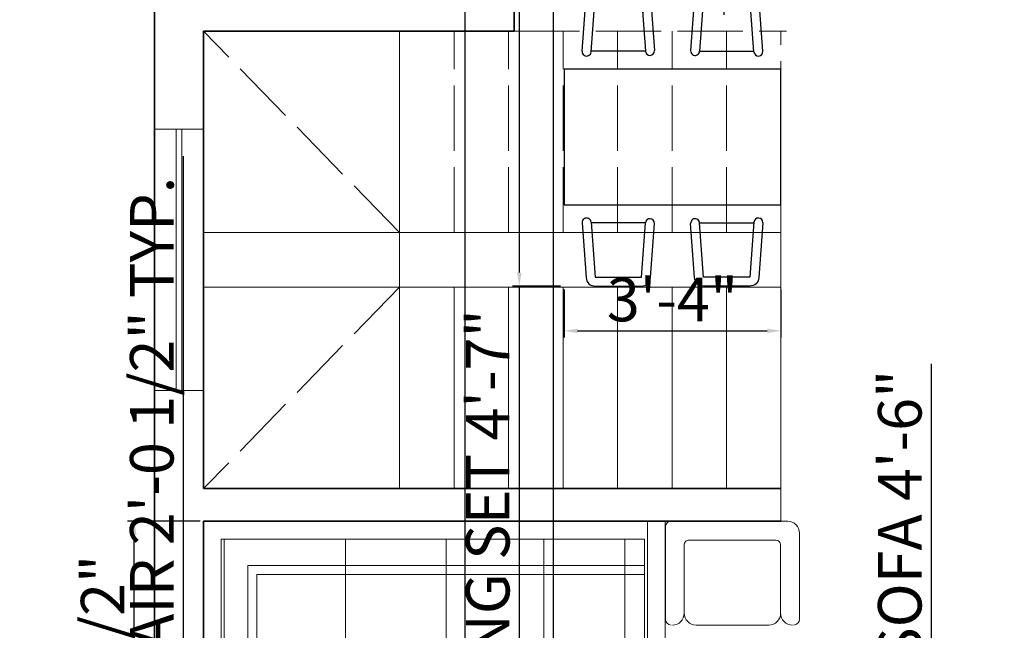
# Model space of a CAD drawing. Units: inches. Extents: x 3394 to 4794, y 965 to 1718.
# Tile 7 of 15: x 3523 to 3704, y 1338 to 1450. Entities that reach past the tile are written whole.
import ezdxf

# ---------------------------------------------------------------- set-up
doc = ezdxf.new("R2010")
doc.units = ezdxf.units.IN
doc.linetypes.add('ACAD_ISO02W100', pattern=[15, 12, -3])
for name, color, linetype, lineweight in [('A-ANNO-DIMS', 2, 'Continuous', 13), ('A-FLOR-STRS', 7, 'Continuous', 18), ('A-FLOR-STRS-OVHD', 7, 'ACAD_ISO02W100', 13), ('A-GLAZ', 4, 'Continuous', 18), ('A-WALL', 7, 'Continuous', 35), ('NOITHAT', 21, 'Continuous', 18)]:
    doc.layers.add(name, color=color, linetype=linetype, lineweight=lineweight)
doc.layers.add('NOI THAT', color=42, linetype='Continuous')
doc.styles.get("Standard").update_dxf_attribs({"font": 'arial.ttf'})
doc.dimstyles.new('ISO-25', dxfattribs={"dimtxt": 8, "dimasz": 2.5, "dimexe": 1.25, "dimexo": 0.625, "dimtad": 1, "dimlunit": 3, "dimtxsty": 'Standard', "dimcen": 2.5, "dimadec": 0, "dimazin": 0, "dimtfac": 1, "dimtmove": 0, "dimatfit": 3, "dimfxl": 1, "dimarcsym": 0})

# ---------------------------------------------------------------- blocks, each defined once
blk = doc.blocks.new('sofa-27')
at = {"color": 0, "linetype": 'ByBlock'}
for p, q in [((0.0945, 0.5198), (0.459, 0.5198)), ((-0.0591, 0.0591), (-0.0591, 0.4902)), ((0.0354, 0.1181), (0.0354, 0.4607)), ((0.518, 0.1181), (0.518, 0.4607)), ((0.6125, 0.0295), (0.6125, 0.4902)), ((0.4944, 0.0945), (0.0591, 0.0945)), ((0.583, 0), (0, 0))]:
    blk.add_line(p, q, dxfattribs=at)
for centre, radius, start, end in [((-0.0295, 0.4902), 0.0295, 90, 180), ((-0.0236, 0.4607), 0.0591, 360, 90), ((0.0945, 0.4607), 0.0591, 90, 180), ((0.459, 0.4607), 0.0591, 0, 90), ((0.5771, 0.4607), 0.0591, 90, 180), ((0.583, 0.4902), 0.0295, 0, 90), ((0.0591, 0.1181), 0.0236, 180, 270), ((0.4944, 0.1181), 0.0236, 270, 0), ((0, 0.0591), 0.0591, 180, 270), ((0.583, 0.0295), 0.0295, 270, 0)]:
    blk.add_arc(centre, radius, start, end, dxfattribs=at)
blk = doc.blocks.new('TABLE-30A')
at = {"color": 0, "linetype": 'ByBlock'}
for p, q in [((0, 0), (0, 0.55)), ((0, 0.55), (1.5, 0.55)), ((1.5, 0.55), (1.5, 0)), ((0.051, 0.508), (0.042, 0.499)), ((0.042, 0.499), (0.042, 0.478)), ((0.042, 0.478), (0.072, 0.478)), ((0.042, 0.478), (0.042, 0.41)), ((0.072, 0.508), (0.051, 0.508)), ((0.051, 0.478), (0.051, 0.41)), ((0.072, 0.478), (0.072, 0.508)), ((0.072, 0.508), (0.14, 0.508)), ((0.072, 0.499), (0.14, 0.499)), ((1.331, 0.508), (0.169, 0.508)), ((1.331, 0.499), (0.169, 0.499)), ((1.428, 0.508), (1.36, 0.508)), ((1.428, 0.499), (1.36, 0.499)), ((1.428, 0.508), (1.428, 0.478)), ((1.449, 0.508), (1.428, 0.508)), ((1.428, 0.478), (1.458, 0.478)), ((1.458, 0.499), (1.449, 0.508)), ((1.449, 0.478), (1.449, 0.41)), ((1.458, 0.478), (1.458, 0.499)), ((1.458, 0.478), (1.458, 0.41)), ((0.042, 0.169), (0.042, 0.381)), ((0.051, 0.169), (0.051, 0.381)), ((1.449, 0.381), (1.449, 0.169)), ((1.458, 0.381), (1.458, 0.169)), ((0.042, 0.072), (0.042, 0.14)), ((0.051, 0.072), (0.051, 0.14)), ((1.449, 0.072), (1.449, 0.14)), ((1.458, 0.072), (1.458, 0.14)), ((1.5, 0), (0, 0)), ((0.042, 0.072), (0.042, 0.051)), ((0.072, 0.072), (0.042, 0.072)), ((0.042, 0.051), (0.051, 0.042)), ((0.051, 0.042), (0.072, 0.042)), ((0.072, 0.042), (0.072, 0.072)), ((0.072, 0.051), (0.14, 0.051)), ((0.072, 0.042), (0.14, 0.042)), ((0.169, 0.051), (1.331, 0.051)), ((0.169, 0.042), (1.331, 0.042)), ((1.428, 0.051), (1.36, 0.051)), ((1.428, 0.042), (1.36, 0.042)), ((1.428, 0.072), (1.428, 0.042)), ((1.458, 0.072), (1.428, 0.072)), ((1.428, 0.042), (1.449, 0.042)), ((1.449, 0.042), (1.458, 0.051)), ((1.458, 0.051), (1.458, 0.072))]:
    blk.add_line(p, q, dxfattribs=at)
blk = doc.blocks.new('12')
at = {"color": 0}
for p, q in [((5656.26, 3021.25), (5553.9, 3021.25)), ((5553.9, 3021.25), (5553.9, 2989.76)), ((5557.83, 3021.25), (5557.83, 2989.76)), ((5656.26, 2989.76), (5656.26, 3021.25)), ((5652.32, 3017.31), (5558.49, 3017.31)), ((5558.49, 3017.31), (5558.49, 2989.76)), ((5562.89, 3017.31), (5562.89, 2989.76)), ((5580.8, 3017.31), (5580.8, 2989.76)), ((5602.45, 3017.31), (5602.45, 2989.76)), ((5624.76, 3017.31), (5624.76, 2954.53)), ((5651.66, 3017.31), (5651.66, 2954.53)), ((5652.32, 2989.76), (5652.32, 3017.31)), ((5646.42, 3011.41), (5558.49, 3011.41)), ((5646.42, 2954.53), (5646.42, 3011.41)), ((5644.45, 3009.44), (5558.49, 3009.44)), ((5644.45, 2954.53), (5644.45, 3009.44)), ((5624.76, 2995), (5624.76, 2954.53)), ((5558.49, 2989.76), (5624.76, 2989.76)), ((5651.66, 2954.53), (5624.76, 2954.53))]:
    blk.add_line(p, q, dxfattribs=at)
for centre in [(5555.86, 2989.76), (5654.29, 2989.76)]:
    blk.add_arc(centre, 1.97, 180, 0, dxfattribs=at)
at = {"xscale": -20.70834898381633, "yscale": 20.70834898381633, "zscale": 20.70834898381633}
blk.add_blockref('TABLE-30A', (5601.8, 2960.82), dxfattribs=at)
blk = doc.blocks.new('A$C02103572')
at = {"layer": 'NOI THAT'}
for p, q in [((450, 1200), (450, 0)), ((1200, 1200), (450, 1200)), ((1200, 0), (1200, 1200)), ((350, 750.1), (350, 1049.9)), ((1300, 750.1), (1300, 1049.9)), ((350, 449.9), (350, 150.1)), ((1300, 449.9), (1300, 150.1)), ((450, 0), (1200, 0))]:
    blk.add_line(p, q, dxfattribs=at)
for points in [[(350, 1100), (46.9, 1077.9, 0.396047), (0, 1028), (0, 772, 0.396047), (46.9, 722.1), (346.4, 700.3)], [(1300, 1100), (1603.1, 1077.9, -0.396047), (1650, 1028), (1650, 772, -0.396047), (1603.1, 722.1), (1303.6, 700.3)], [(350, 100), (46.9, 122.1, -0.396047), (0, 172), (0, 428, -0.396047), (46.9, 477.9), (346.4, 499.7)], [(1300, 100), (1603.1, 122.1, 0.396047), (1650, 172), (1650, 428, 0.396047), (1603.1, 477.9), (1303.6, 499.7)]]:
    blk.add_lwpolyline(points, format="xyb", dxfattribs=at)
for points in [[(353.6, 1050.1), (50, 1028), (50, 772), (350, 750.1)], [(1296.4, 1050.1), (1600, 1028), (1600, 772), (1300, 750.1)], [(353.6, 149.9), (50, 172), (50, 428), (350, 449.9)], [(1296.4, 149.9), (1600, 172), (1600, 428), (1300, 449.9)]]:
    blk.add_lwpolyline(points, dxfattribs=at)
for centre, start, end in [((351.8, 1075.1), 274.1643, 94.1643), ((1298.2, 1075.1), 85.8357, 265.8357), ((348.2, 725.2), 265.8357, 85.8357), ((1301.8, 725.2), 94.1643, 274.1643), ((348.2, 474.8), 274.1643, 94.1643), ((1301.8, 474.8), 85.8357, 265.8357), ((351.8, 124.9), 265.8357, 85.8357), ((1298.2, 124.9), 94.1643, 274.1643)]:
    blk.add_arc(centre, 25, start, end, dxfattribs=at)
blk = doc.blocks.new('WIN-48IN')
for p, q in [((9, 48), (0, 48)), ((4, 0), (4, 48)), ((5, 0), (5, 48)), ((9, 0), (0, 0))]:
    blk.add_line(p, q)
blk = doc.blocks.new('*D76')
at = {"layer": 'A-ANNO-DIMS', "color": 0, "lineweight": -2, "transparency": 16777216}
for p, q in [((3553.05, 1290.42), (3553.05, 1424.75)), ((3556.12, 1290.42), (3551.8, 1290.42)), ((3553.05, 1268.3), (3553.05, 1287.92)), ((3556.12, 1265.8), (3551.8, 1265.8))]:
    blk.add_line(p, q, dxfattribs=at)
at = {"layer": 'A-ANNO-DIMS', "color": 0, "transparency": 16777216}
for points in [[(3552.63, 1287.92), (3553.47, 1287.92), (3553.05, 1290.42)], [(3552.63, 1268.3), (3553.47, 1268.3), (3553.05, 1265.8)]]:
    blk.add_solid(points, dxfattribs=at)
at = {"layer": 'Defpoints', "color": 0, "transparency": 16777216}
for p in [(3553.05, 1290.42), (3556.74, 1290.42), (3556.74, 1265.8)]:
    blk.add_point(p, dxfattribs=at)
at = {"layer": 'A-ANNO-DIMS', "color": 0, "transparency": 16777216, "insert": (3548.29, 1358.84), "char_height": 8, "attachment_point": 5, "rotation": 90}
blk.add_mtext('ARMCHAIR 2\'-0 1/2" TYP.', dxfattribs=at)
blk = doc.blocks.new('*D88')
at = {"layer": 'A-ANNO-DIMS', "color": 0, "lineweight": -2, "transparency": 16777216}
for p, q in [((3637.38, 1453.56), (3637.38, 1450.71)), ((3652.23, 1453.56), (3652.23, 1450.7)), ((3639.88, 1451.96), (3649.73, 1451.96)), ((3652.23, 1451.95), (3745.7, 1451.93))]:
    blk.add_line(p, q, dxfattribs=at)
at = {"layer": 'A-ANNO-DIMS', "color": 0, "transparency": 16777216}
for points in [[(3639.88, 1452.37), (3639.88, 1451.54), (3637.38, 1451.96)], [(3649.73, 1452.37), (3649.73, 1451.54), (3652.23, 1451.95)]]:
    blk.add_solid(points, dxfattribs=at)
at = {"layer": 'Defpoints', "color": 0, "transparency": 16777216}
for p in [(3637.38, 1454.19), (3652.23, 1454.18), (3652.23, 1451.95)]:
    blk.add_point(p, dxfattribs=at)
at = {"layer": 'A-ANNO-DIMS', "color": 0, "transparency": 16777216, "insert": (3700.21, 1456.71), "char_height": 8, "attachment_point": 5, "rotation": 359.9851}
blk.add_mtext('STOOL 1\'-3" TYP.', dxfattribs=at)
blk = doc.blocks.new('*D101')
at = {"layer": 'A-ANNO-DIMS', "color": 0, "lineweight": -2, "transparency": 16777216}
for p, q in [((3556.12, 1357.68), (3542.78, 1357.68)), ((3544.03, 1304.92), (3544.03, 1355.18)), ((3556.12, 1302.42), (3542.78, 1302.42))]:
    blk.add_line(p, q, dxfattribs=at)
at = {"layer": 'A-ANNO-DIMS', "color": 0, "transparency": 16777216}
for points in [[(3543.61, 1355.18), (3544.44, 1355.18), (3544.03, 1357.68)], [(3543.61, 1304.92), (3544.44, 1304.92), (3544.03, 1302.42)]]:
    blk.add_solid(points, dxfattribs=at)
at = {"layer": 'Defpoints', "color": 0, "transparency": 16777216}
for p in [(3544.03, 1357.68), (3556.74, 1357.68), (3556.74, 1302.42)]:
    blk.add_point(p, dxfattribs=at)
at = {"layer": 'A-ANNO-DIMS', "color": 0, "transparency": 16777216, "insert": (3539.27, 1330.05), "char_height": 8, "attachment_point": 5, "rotation": 90}
blk.add_mtext('4\'-7 1/2"', dxfattribs=at)
blk = doc.blocks.new('*D102')
at = {"layer": 'A-ANNO-DIMS', "color": 0, "lineweight": -2, "transparency": 16777216}
for p, q in [((3690.36, 1328.09), (3690.36, 1386.6)), ((3697.86, 1328.09), (3689.11, 1328.09)), ((3690.36, 1276.43), (3690.36, 1325.59)), ((3697.86, 1273.93), (3689.11, 1273.93))]:
    blk.add_line(p, q, dxfattribs=at)
at = {"layer": 'A-ANNO-DIMS', "color": 0, "transparency": 16777216}
for points in [[(3689.94, 1325.59), (3690.77, 1325.59), (3690.36, 1328.09)], [(3689.94, 1276.43), (3690.77, 1276.43), (3690.36, 1273.93)]]:
    blk.add_solid(points, dxfattribs=at)
at = {"layer": 'Defpoints', "color": 0, "transparency": 16777216}
for p in [(3690.36, 1328.09), (3698.48, 1328.09), (3698.48, 1273.93)]:
    blk.add_point(p, dxfattribs=at)
at = {"layer": 'A-ANNO-DIMS', "color": 0, "transparency": 16777216, "insert": (3685.59, 1358.6), "char_height": 8, "attachment_point": 5, "rotation": 90}
blk.add_mtext('SOFA 4\'-6"', dxfattribs=at)
blk = doc.blocks.new('*D104')
at = {"layer": 'A-ANNO-DIMS', "color": 0, "lineweight": -2, "transparency": 16777216}
for p, q in [((3622.3, 1455.61), (3613.46, 1455.61)), ((3614.71, 1453.11), (3614.71, 1403.36)), ((3622.3, 1400.86), (3613.46, 1400.86)), ((3614.71, 1400.86), (3614.71, 1309.18))]:
    blk.add_line(p, q, dxfattribs=at)
at = {"layer": 'A-ANNO-DIMS', "color": 0, "transparency": 16777216}
for points in [[(3614.29, 1453.11), (3615.13, 1453.11), (3614.71, 1455.61)], [(3614.29, 1403.36), (3615.13, 1403.36), (3614.71, 1400.86)]]:
    blk.add_solid(points, dxfattribs=at)
at = {"layer": 'Defpoints', "color": 0, "transparency": 16777216}
for p in [(3622.92, 1455.61), (3614.71, 1400.86), (3622.92, 1400.86)]:
    blk.add_point(p, dxfattribs=at)
at = {"layer": 'A-ANNO-DIMS', "color": 0, "transparency": 16777216, "insert": (3609.95, 1353.77), "char_height": 8, "attachment_point": 5, "rotation": 90}
blk.add_mtext('DINING SET 4\'-7"', dxfattribs=at)
blk = doc.blocks.new('*D105')
at = {"layer": 'A-ANNO-DIMS', "color": 0, "lineweight": -2, "transparency": 16777216}
for p, q in [((3622.92, 1400.23), (3622.92, 1391.4)), ((3662.74, 1400.23), (3662.74, 1391.4)), ((3625.42, 1392.65), (3660.24, 1392.65))]:
    blk.add_line(p, q, dxfattribs=at)
at = {"layer": 'A-ANNO-DIMS', "color": 0, "transparency": 16777216}
for points in [[(3625.42, 1393.06), (3625.42, 1392.23), (3622.92, 1392.65)], [(3660.24, 1393.06), (3660.24, 1392.23), (3662.74, 1392.65)]]:
    blk.add_solid(points, dxfattribs=at)
at = {"layer": 'Defpoints', "color": 0, "transparency": 16777216}
for p in [(3622.92, 1400.86), (3662.74, 1400.86), (3662.74, 1392.65)]:
    blk.add_point(p, dxfattribs=at)
at = {"layer": 'A-ANNO-DIMS', "color": 0, "transparency": 16777216, "insert": (3642.83, 1397.36), "char_height": 8, "attachment_point": 5}
blk.add_mtext('3\'-4"', dxfattribs=at)
blk = doc.blocks.new('*D123')
at = {"layer": 'A-ANNO-DIMS', "color": 0, "lineweight": -2, "transparency": 16777216}
for p, q in [((3604.74, 1582.06), (3604.74, 987.36)), ((3620.92, 1582.06), (3620.92, 987.36)), ((3607.24, 988.61), (3618.42, 988.61)), ((3620.92, 988.61), (3645.18, 988.61))]:
    blk.add_line(p, q, dxfattribs=at)
at = {"layer": 'A-ANNO-DIMS', "color": 0, "transparency": 16777216}
for points in [[(3607.24, 989.03), (3607.24, 988.2), (3604.74, 988.61)], [(3618.42, 989.03), (3618.42, 988.2), (3620.92, 988.61)]]:
    blk.add_solid(points, dxfattribs=at)
at = {"layer": 'Defpoints', "color": 0, "transparency": 16777216}
for p in [(3604.74, 1582.68), (3620.92, 1582.68), (3620.92, 988.61)]:
    blk.add_point(p, dxfattribs=at)
at = {"layer": 'A-ANNO-DIMS', "color": 0, "transparency": 16777216, "insert": (3634.3, 993.25), "char_height": 8, "attachment_point": 5}
blk.add_mtext('1\'-4"', dxfattribs=at)

msp = doc.modelspace()

# ---------------------------------------------------------------- linework, layer by layer
at = {"layer": 'A-FLOR-STRS'}
for p, q in [((3592.745, 1363.682), (3592.745, 1447.682)), ((3662.745, 1357.682), (3662.745, 1415.182)), ((3556.745, 1410.682), (3662.745, 1410.682)), ((3556.745, 1400.682), (3662.745, 1400.682)), ((3602.745, 1363.682), (3602.745, 1400.682)), ((3612.745, 1363.682), (3612.745, 1400.682)), ((3622.745, 1363.682), (3622.745, 1400.682)), ((3632.745, 1363.682), (3632.745, 1400.682)), ((3642.745, 1363.682), (3642.745, 1400.682)), ((3652.745, 1363.682), (3652.745, 1400.682))]:
    msp.add_line(p, q, dxfattribs=at)
at = {"layer": 'A-FLOR-STRS-OVHD'}
for p, q in [((3592.745, 1410.682), (3556.745, 1447.682)), ((3602.745, 1410.682), (3602.745, 1447.682)), ((3612.745, 1410.682), (3612.745, 1447.682)), ((3613.745, 1447.682), (3663.745, 1447.682)), ((3622.745, 1410.682), (3622.745, 1447.682)), ((3632.745, 1410.682), (3632.745, 1447.682)), ((3642.745, 1410.682), (3642.745, 1447.682)), ((3652.745, 1410.682), (3652.745, 1447.682)), ((3662.745, 1415.182), (3662.745, 1447.682)), ((3592.745, 1400.682), (3556.745, 1363.682))]:
    msp.add_line(p, q, dxfattribs=at)
at = {"layer": 'A-WALL'}
for p, q in [((3613.745, 1573.682), (3613.745, 1447.682)), ((3547.745, 1117.682), (3547.745, 1456.682)), ((3556.745, 1447.682), (3613.745, 1447.682)), ((3556.745, 1363.682), (3556.745, 1447.682)), ((3556.745, 1363.682), (3662.745, 1363.682)), ((3556.745, 1207.682), (3556.745, 1357.682)), ((3556.745, 1357.682), (3662.745, 1357.682))]:
    msp.add_line(p, q, dxfattribs=at)

# ---------------------------------------------------------------- block references
at = {"layer": 'A-GLAZ'}
msp.add_blockref('WIN-48IN', (3547.745, 1381.682), dxfattribs=at)
at = {"layer": 'NOITHAT'}
for name, p, xscale, yscale, zscale, rotation in [('A$C02103572', (3622.924, 1455.611), 0.033183731328394, 0.033183731328394, 0.033183731328394, 270), ('sofa-27', (3663.981, 1357.682), 36.66436083614781, 36.66436083614781, 36.66436083614781, 180)]:
    msp.add_blockref(name, p, dxfattribs=dict(at, xscale=xscale, yscale=yscale, zscale=zscale, rotation=rotation))
at = {"layer": 'NOITHAT', "xscale": -0.8282073146500575, "yscale": 0.8282073146500575, "zscale": 0.8282073146500575}
msp.add_blockref('12', (8241.3, -1144.54), dxfattribs=at)

# ---------------------------------------------------------------- dimensions: what is measured, and where the dimension line sits
at = {"layer": 'A-ANNO-DIMS'}
for base, p1, p2, picture, middle in [((3620.921, 988.612), (3604.745, 1582.682), (3620.921, 1582.682), '*D123', (3634.302, 993.254)), ((3662.745, 1392.645), (3622.924, 1400.858), (3662.745, 1400.858), '*D105', (3642.834, 1397.357))]:
    dim = msp.add_linear_dim(base=base, p1=p1, p2=p2, dimstyle='ISO-25', override={"dimdec": 1, "dimlfac": 1, "dimrnd": 0, "dimzin": 1, "dimdsep": 46, "dimlunit": 4, "dimfrac": 2}, dxfattribs=at)
    dim.commit()
    dim.dimension.update_dxf_attribs({"geometry": picture, "text_midpoint": middle})
for base, p1, p2, angle, text, picture, middle in [((3652.232, 1451.955), (3637.379, 1454.186), (3652.232, 1454.183), 359.9851, 'STOOL <> TYP.', '*D88', (3700.215, 1456.709)), ((3614.711, 1400.858), (3622.924, 1455.611), (3622.924, 1400.858), 270, 'DINING SET <>', '*D104', (3609.95, 1353.769)), ((3553.051, 1290.42), (3556.745, 1265.797), (3556.745, 1290.42), 90, 'ARMCHAIR <> TYP.', '*D76', (3548.29, 1358.835)), ((3690.358, 1328.093), (3698.483, 1273.927), (3698.483, 1328.093), 90, 'SOFA <>', '*D102', (3685.593, 1358.599))]:
    dim = msp.add_linear_dim(base=base, p1=p1, p2=p2, angle=angle, text=text, dimstyle='ISO-25', override={"dimdec": 1, "dimlfac": 1, "dimrnd": 0, "dimzin": 1, "dimdsep": 46, "dimlunit": 4, "dimfrac": 2}, dxfattribs=at)
    dim.commit()
    dim.dimension.update_dxf_attribs({"geometry": picture, "text_midpoint": middle})
dim = msp.add_linear_dim(base=(3544.028, 1357.682), p1=(3556.745, 1302.42), p2=(3556.745, 1357.682), angle=90, dimstyle='ISO-25', override={"dimdec": 1, "dimlfac": 1, "dimrnd": 0, "dimzin": 1, "dimdsep": 46, "dimlunit": 4, "dimfrac": 2}, dxfattribs=at)
dim.commit()
dim.dimension.update_dxf_attribs({"geometry": '*D101', "text_midpoint": (3539.267, 1330.051)})

doc.saveas('drawing.dxf')
